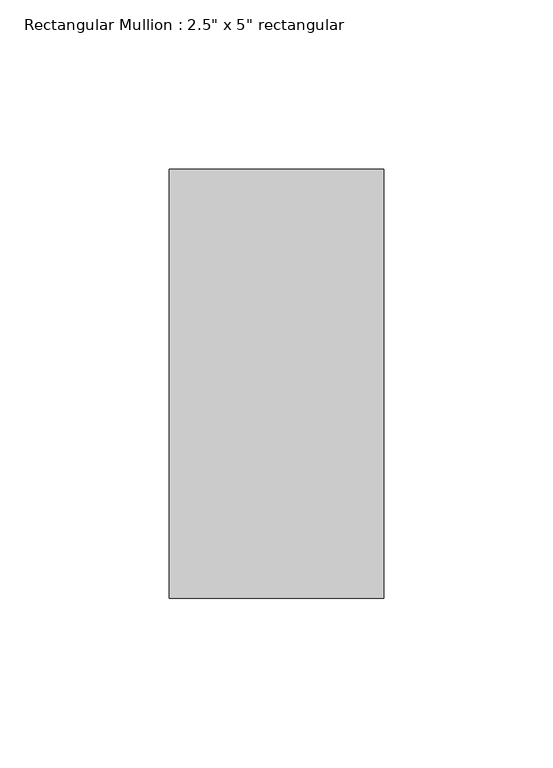
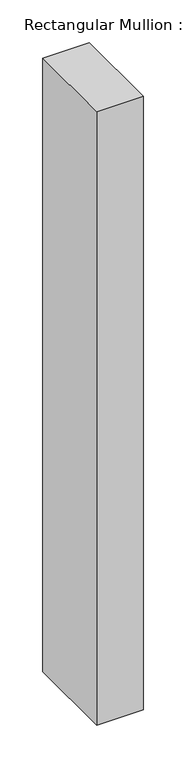
"""IFC4 building model written with IfcOpenShell, lengths in millimetres: member geometry."""

from ifc_helpers import new_model, si_unit, frame, origin, place, context, project, spatial, polyline, outline, extrude, source, transform, mapped, element, save


def member_8834d53d(model_context):
    return source(origin(), model_context, "Body", "SweptSolid", [
        extrude(outline(polyline([(0.0, 63.5), (0.0, -63.5), (-63.5, -63.5), (-63.5, 63.5), (0.0, 63.5)])), frame((0.0, 0.0, -880.5333333), z_axis=(0.0, 0.0, 1.0), x_axis=(1.0, 0.0, 0.0)), (0.0, 0.0, 1.0), 880.5333333),
    ])


if __name__ == "__main__":
    model = new_model("IFC4")
    model_context = context("Model", 3, world=origin())
    ifc_project = project(units=[si_unit("LENGTHUNIT", "METRE", prefix="MILLI")], contexts=[model_context])
    site = spatial("IfcSite", under=ifc_project)
    building = spatial("IfcBuilding", under=site)
    placement = place(None, origin())
    member_shape = member_8834d53d(model_context)
    element("IfcMember", 1, ObjectType="Rectangular Mullion : 2.5\" x 5\" rectangular", at=placement, inside=building, context=model_context, shape_type="MappedRepresentation", body=[
        mapped(member_shape, transform((0.0, 0.0, 0.0), x_axis=(1.0, 0.0, 0.0), y_axis=(0.0, 1.0, 0.0), z_axis=(0.0, 0.0, 1.0))),
    ])
    save(model, "model.ifc")

# Revit data of these elements
# Type "Rectangular Mullion : 2.5\" x 5\" rectangular"
#   built-in parameter 1007304 = 0.416667 (stored number, unit not read)
#   built-in parameter 1007301 = 0.104167 (stored number, unit not read)
#   built-in parameter 1007300 = 0.104167 (stored number, unit not read)
# Element 1 (IfcMember, "Rectangular Mullion : 2.5\" x 5\" rectangular")
#   Materials on its faces: "Aluminum"
# Materials
#   "Aluminum": class "Metal", colour RGB 247 247 247, transparency 0, Description = "Aluminum 6061", Cost = 0
